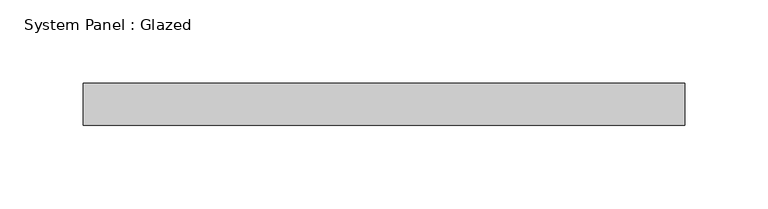
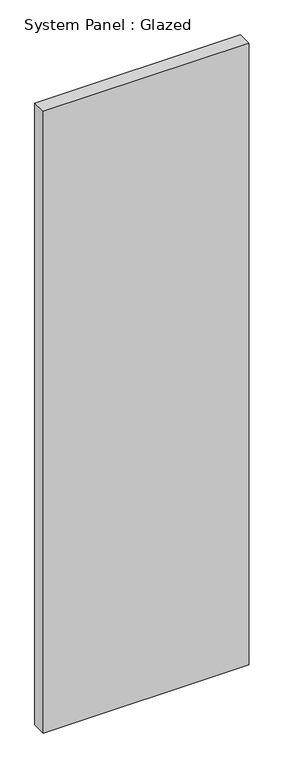
"""IFC4 building model written with IfcOpenShell, lengths in millimetres: plate geometry, System Panel : Glazed."""

from ifc_helpers import new_model, si_unit, origin, origin_with_axes, place, context, project, spatial, polyline, outline, extrude, source, transform, mapped, element, save


def system_panel_glazed_28d38409(model_context):
    return source(origin(), model_context, "Body", "SweptSolid", [
        extrude(outline(polyline([(180.975, 19.05), (-180.975, 19.05), (-180.975, 44.45), (180.975, 44.45), (180.975, 19.05)])), origin_with_axes(), (0.0, 0.0, 1.0), 1155.7),
    ])


if __name__ == "__main__":
    model = new_model("IFC4")
    model_context = context("Model", 3, world=origin())
    ifc_project = project(units=[si_unit("LENGTHUNIT", "METRE", prefix="MILLI")], contexts=[model_context])
    site = spatial("IfcSite", under=ifc_project)
    building = spatial("IfcBuilding", under=site)
    placement = place(None, origin())
    system_panel_glazed_shape = system_panel_glazed_28d38409(model_context)
    element("IfcPlate", 1, ObjectType="System Panel : Glazed", at=placement, inside=building, context=model_context, shape_type="MappedRepresentation", body=[
        mapped(system_panel_glazed_shape, transform((0.0, 0.0, 0.0), x_axis=(1.0, 0.0, 0.0), y_axis=(0.0, 1.0, 0.0), z_axis=(0.0, 0.0, 1.0))),
    ])
    save(model, "model.ifc")

# Revit data of these elements
# Type "System Panel : Glazed"
#   Construction Type Id = "GSP4R"
#   Analytic Construction = "1/8 in Pilkington single glazing"
#   Visual Light Transmittance = 0.9
#   Solar Heat Gain Coefficient = 0.86
#   Heat Transfer Coefficient (U) = 1.18115 BTU/(h·ft²·°F)
#   Define Thermal Properties by = 1
# Element 1 (IfcPlate, "System Panel : Glazed")
#   Materials on its faces: "Glass"
# Materials
#   "Glass": class "Glass", colour RGB 0 128 192, transparency 0.75, Description = "Soda Lime Glass", Cost = 0
